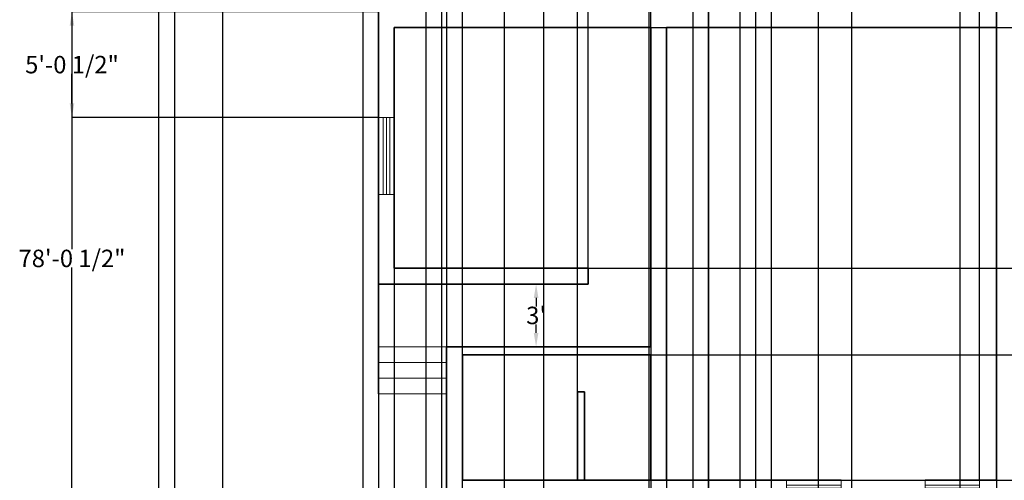
# Model space of a CAD drawing. Units: inches. Extents: x -63 to 800, y 3068 to 4133.
# Tile 2 of 5: x -63 to 501, y 3473 to 3737. Entities that reach past the tile are written whole.
import ezdxf

# ---------------------------------------------------------------- set-up
doc = ezdxf.new("R2010")
doc.units = ezdxf.units.IN
doc.header["$MEASUREMENT"] = 0
for name, color, linetype, lineweight in [('A-ANNO-DIMS', 2, 'Continuous', 13), ('A-FLOR-STRS', 3, 'Continuous', 18), ('A-GLAZ', 4, 'Continuous', 18), ('A-WALL', 7, 'Continuous', 35), ('A-WALL-SITE', 8, 'Continuous', 30)]:
    doc.layers.add(name, color=color, linetype=linetype, lineweight=lineweight)
doc.styles.get("Standard").update_dxf_attribs({"font": 'arial.ttf'})
doc.dimstyles.get("Standard").update_dxf_attribs({"dimtxt": 10, "dimasz": 8, "dimexe": 0.18, "dimexo": 0.0625, "dimgap": 0.09, "dimtad": 0, "dimtih": 1, "dimtoh": 1, "dimdec": 0, "dimzin": 0, "dimdsep": 46, "dimlunit": 3, "dimtxsty": 'Standard', "dimcen": 0.09, "dimadec": 0, "dimazin": 0, "dimtfac": 1, "dimtdec": 0, "dimtofl": 0, "dimtmove": 0, "dimatfit": 3, "dimfxl": 1, "dimtolj": 1, "dimtzin": 0, "dimarcsym": 0})

# ---------------------------------------------------------------- blocks, each defined once
blk = doc.blocks.new('*D6')
at = {"layer": 'A-ANNO-DIMS', "color": 0, "lineweight": -2, "transparency": 16777216}
for p, q in [((224.87, 3585.81), (232.74, 3585.81)), ((232.56, 3577.81), (232.56, 3573.01)), ((232.56, 3557.81), (232.56, 3562.61)), ((224.87, 3549.81), (232.74, 3549.81))]:
    blk.add_line(p, q, dxfattribs=at)
at = {"layer": 'A-ANNO-DIMS', "color": 0, "transparency": 16777216}
for points in [[(231.22, 3577.81), (233.89, 3577.81), (232.56, 3585.81)], [(231.22, 3557.81), (233.89, 3557.81), (232.56, 3549.81)]]:
    blk.add_solid(points, dxfattribs=at)
at = {"layer": 'Defpoints', "color": 0, "transparency": 16777216}
for p in [(224.81, 3585.81), (224.81, 3549.81), (232.56, 3549.81)]:
    blk.add_point(p, dxfattribs=at)
at = {"layer": 'A-ANNO-DIMS', "color": 0, "transparency": 16777216, "insert": (232.56, 3567.81), "char_height": 10, "attachment_point": 5}
blk.add_mtext("\\A1;3'", dxfattribs=at)
blk = doc.blocks.new('WIN-31')
blk.add_lwpolyline([(0, 9), (31.17, 9), (31.17, 0), (0, 0)], close=True)
blk.add_lwpolyline([(0, 4.5), (31.17, 4.5), (31.17, 6.29), (0, 6.29), (0, 2.51), (31.17, 2.51)])
blk = doc.blocks.new('WIN-44')
blk.add_lwpolyline([(0, 0), (0, 44.17), (9, 44.17), (9, 0)], close=True)
for points in [[(2.71, 44.17), (2.71, 0), (6.5, 0), (6.5, 44.17)], [(4.5, 0), (4.5, 44.17)]]:
    blk.add_lwpolyline(points)
blk = doc.blocks.new('*D20')
at = {"layer": 'A-ANNO-DIMS', "color": 0, "lineweight": -2, "transparency": 16777216}
for p, q in [((16.25, 4068.66), (-33.52, 4068.66)), ((-33.34, 4060.66), (-33.34, 3605.75)), ((-33.34, 3140.31), (-33.34, 3595.23)), ((16.25, 3132.31), (-33.52, 3132.31))]:
    blk.add_line(p, q, dxfattribs=at)
at = {"layer": 'A-ANNO-DIMS', "color": 0, "transparency": 16777216}
for points in [[(-34.67, 4060.66), (-32.01, 4060.66), (-33.34, 4068.66)], [(-34.67, 3140.31), (-32.01, 3140.31), (-33.34, 3132.31)]]:
    blk.add_solid(points, dxfattribs=at)
at = {"layer": 'Defpoints', "color": 0, "transparency": 16777216}
for p in [(-33.34, 4068.66), (16.31, 4068.66), (16.31, 3132.31)]:
    blk.add_point(p, dxfattribs=at)
at = {"layer": 'A-ANNO-DIMS', "color": 0, "transparency": 16777216, "insert": (-33.34, 3600.49), "char_height": 10, "attachment_point": 5}
blk.add_mtext('\\A1;78\'-0 1/2"', dxfattribs=at)
blk = doc.blocks.new('*D23')
at = {"layer": 'A-ANNO-DIMS', "color": 0, "lineweight": -2, "transparency": 16777216}
for p, q in [((25.31, 4059.6), (25.31, 3082.48)), ((169.31, 4059.6), (169.31, 3082.48)), ((33.31, 3082.66), (80.51, 3082.66)), ((161.31, 3082.66), (114.1, 3082.66))]:
    blk.add_line(p, q, dxfattribs=at)
at = {"layer": 'A-ANNO-DIMS', "color": 0, "transparency": 16777216}
for points in [[(33.31, 3083.99), (33.31, 3081.33), (25.31, 3082.66)], [(161.31, 3083.99), (161.31, 3081.33), (169.31, 3082.66)]]:
    blk.add_solid(points, dxfattribs=at)
at = {"layer": 'Defpoints', "color": 0, "transparency": 16777216}
for p in [(25.31, 4059.66), (169.31, 4059.66), (169.31, 3082.66)]:
    blk.add_point(p, dxfattribs=at)
at = {"layer": 'A-ANNO-DIMS', "color": 0, "transparency": 16777216, "insert": (97.31, 3082.66), "char_height": 10, "attachment_point": 5}
blk.add_mtext('\\A1;12\'-0"', dxfattribs=at)
blk = doc.blocks.new('*D24')
at = {"layer": 'A-ANNO-DIMS', "color": 0, "lineweight": -2, "transparency": 16777216}
for p, q in [((178.31, 4059.6), (178.31, 3082.48)), ((322.31, 4059.6), (322.31, 3082.48)), ((186.31, 3082.66), (233.51, 3082.66)), ((314.31, 3082.66), (267.1, 3082.66))]:
    blk.add_line(p, q, dxfattribs=at)
at = {"layer": 'A-ANNO-DIMS', "color": 0, "transparency": 16777216}
for points in [[(186.31, 3083.99), (186.31, 3081.33), (178.31, 3082.66)], [(314.31, 3083.99), (314.31, 3081.33), (322.31, 3082.66)]]:
    blk.add_solid(points, dxfattribs=at)
at = {"layer": 'Defpoints', "color": 0, "transparency": 16777216}
for p in [(178.31, 4059.66), (322.31, 4059.66), (322.31, 3082.66)]:
    blk.add_point(p, dxfattribs=at)
at = {"layer": 'A-ANNO-DIMS', "color": 0, "transparency": 16777216, "insert": (250.31, 3082.66), "char_height": 10, "attachment_point": 5}
blk.add_mtext('\\A1;12\'-0"', dxfattribs=at)
blk = doc.blocks.new('*D25')
at = {"layer": 'A-ANNO-DIMS', "color": 0, "lineweight": -2, "transparency": 16777216}
for p, q in [((331.31, 4059.6), (331.31, 3082.48)), ((475.31, 4059.6), (475.31, 3082.48)), ((339.31, 3082.66), (386.51, 3082.66)), ((467.31, 3082.66), (420.1, 3082.66))]:
    blk.add_line(p, q, dxfattribs=at)
at = {"layer": 'A-ANNO-DIMS', "color": 0, "transparency": 16777216}
for points in [[(339.31, 3083.99), (339.31, 3081.33), (331.31, 3082.66)], [(467.31, 3083.99), (467.31, 3081.33), (475.31, 3082.66)]]:
    blk.add_solid(points, dxfattribs=at)
at = {"layer": 'Defpoints', "color": 0, "transparency": 16777216}
for p in [(331.31, 4059.66), (475.31, 4059.66), (475.31, 3082.66)]:
    blk.add_point(p, dxfattribs=at)
at = {"layer": 'A-ANNO-DIMS', "color": 0, "transparency": 16777216, "insert": (403.31, 3082.66), "char_height": 10, "attachment_point": 5}
blk.add_mtext('\\A1;12\'-0"', dxfattribs=at)
blk = doc.blocks.new('*D27')
at = {"layer": 'A-ANNO-DIMS', "color": 0, "lineweight": -2, "transparency": 16777216}
for p, q in [((25.31, 3951.6), (25.31, 3082.48)), ((52.97, 3951.6), (52.97, 3082.48)), ((33.31, 3082.66), (44.97, 3082.66)), ((52.97, 3082.66), (60.97, 3082.66))]:
    blk.add_line(p, q, dxfattribs=at)
at = {"layer": 'A-ANNO-DIMS', "color": 0, "transparency": 16777216}
for points in [[(33.31, 3083.99), (33.31, 3081.33), (25.31, 3082.66)], [(44.97, 3083.99), (44.97, 3081.33), (52.97, 3082.66)]]:
    blk.add_solid(points, dxfattribs=at)
at = {"layer": 'Defpoints', "color": 0, "transparency": 16777216}
for p in [(25.31, 3951.66), (52.97, 3951.66), (52.97, 3082.66)]:
    blk.add_point(p, dxfattribs=at)
at = {"layer": 'A-ANNO-DIMS', "color": 0, "transparency": 16777216, "insert": (86.08, 3082.66), "char_height": 10, "attachment_point": 5}
blk.add_mtext('\\A1;2\'-3 1/2"', dxfattribs=at)
blk = doc.blocks.new('*D28')
at = {"layer": 'A-ANNO-DIMS', "color": 0, "lineweight": -2, "transparency": 16777216}
for p, q in [((297.16, 3951.55), (297.16, 3082.48)), ((331.31, 3951.6), (331.31, 3082.48)), ((305.16, 3082.66), (323.31, 3082.66)), ((331.31, 3082.66), (339.31, 3082.66))]:
    blk.add_line(p, q, dxfattribs=at)
at = {"layer": 'A-ANNO-DIMS', "color": 0, "transparency": 16777216}
for points in [[(305.16, 3083.99), (305.16, 3081.33), (297.16, 3082.66)], [(323.31, 3083.99), (323.31, 3081.33), (331.31, 3082.66)]]:
    blk.add_solid(points, dxfattribs=at)
at = {"layer": 'Defpoints', "color": 0, "transparency": 16777216}
for p in [(297.16, 3951.61), (331.31, 3951.66), (331.31, 3082.66)]:
    blk.add_point(p, dxfattribs=at)
at = {"layer": 'A-ANNO-DIMS', "color": 0, "transparency": 16777216, "insert": (356.66, 3082.66), "char_height": 10, "attachment_point": 5}
blk.add_mtext('\\A1;2\'-10"', dxfattribs=at)
blk = doc.blocks.new('*D29')
at = {"layer": 'A-ANNO-DIMS', "color": 0, "lineweight": -2, "transparency": 16777216}
for p, q in [((367.31, 3951.6), (367.31, 3082.48)), ((413.21, 3951.6), (413.21, 3082.48)), ((359.31, 3082.66), (351.31, 3082.66)), ((421.21, 3082.66), (429.21, 3082.66))]:
    blk.add_line(p, q, dxfattribs=at)
at = {"layer": 'A-ANNO-DIMS', "color": 0, "transparency": 16777216}
for points in [[(359.31, 3083.99), (359.31, 3081.33), (367.31, 3082.66)], [(421.21, 3083.99), (421.21, 3081.33), (413.21, 3082.66)]]:
    blk.add_solid(points, dxfattribs=at)
at = {"layer": 'Defpoints', "color": 0, "transparency": 16777216}
for p in [(367.31, 3951.66), (413.21, 3951.66), (413.21, 3082.66)]:
    blk.add_point(p, dxfattribs=at)
at = {"layer": 'A-ANNO-DIMS', "color": 0, "transparency": 16777216, "insert": (390.26, 3082.66), "char_height": 10, "attachment_point": 5}
blk.add_mtext('\\A1;3\'-10"', dxfattribs=at)
blk = doc.blocks.new('*D30')
at = {"layer": 'A-ANNO-DIMS', "color": 0, "lineweight": -2, "transparency": 16777216}
for p, q in [((133.31, 3951.6), (133.31, 3082.48)), ((169.31, 3951.6), (169.31, 3082.48)), ((125.31, 3082.66), (117.31, 3082.66)), ((177.31, 3082.66), (185.31, 3082.66))]:
    blk.add_line(p, q, dxfattribs=at)
at = {"layer": 'A-ANNO-DIMS', "color": 0, "transparency": 16777216}
for points in [[(125.31, 3083.99), (125.31, 3081.33), (133.31, 3082.66)], [(177.31, 3083.99), (177.31, 3081.33), (169.31, 3082.66)]]:
    blk.add_solid(points, dxfattribs=at)
at = {"layer": 'Defpoints', "color": 0, "transparency": 16777216}
for p in [(133.31, 3951.66), (169.31, 3951.66), (169.31, 3082.66)]:
    blk.add_point(p, dxfattribs=at)
at = {"layer": 'A-ANNO-DIMS', "color": 0, "transparency": 16777216, "insert": (151.31, 3082.66), "char_height": 10, "attachment_point": 5}
blk.add_mtext('\\A1;3\'-0"', dxfattribs=at)
blk = doc.blocks.new('*D31')
at = {"layer": 'A-ANNO-DIMS', "color": 0, "lineweight": -2, "transparency": 16777216}
for p, q in [((178.31, 3951.6), (178.31, 3082.48)), ((214.31, 3951.6), (214.31, 3082.48)), ((170.31, 3082.66), (162.31, 3082.66)), ((222.31, 3082.66), (230.31, 3082.66))]:
    blk.add_line(p, q, dxfattribs=at)
at = {"layer": 'A-ANNO-DIMS', "color": 0, "transparency": 16777216}
for points in [[(170.31, 3083.99), (170.31, 3081.33), (178.31, 3082.66)], [(222.31, 3083.99), (222.31, 3081.33), (214.31, 3082.66)]]:
    blk.add_solid(points, dxfattribs=at)
at = {"layer": 'Defpoints', "color": 0, "transparency": 16777216}
for p in [(178.31, 3951.66), (214.31, 3951.66), (214.31, 3082.66)]:
    blk.add_point(p, dxfattribs=at)
at = {"layer": 'A-ANNO-DIMS', "color": 0, "transparency": 16777216, "insert": (196.31, 3082.66), "char_height": 10, "attachment_point": 5}
blk.add_mtext('\\A1;3\'-0"', dxfattribs=at)
blk = doc.blocks.new('*D32')
at = {"layer": 'A-ANNO-DIMS', "color": 0, "lineweight": -2, "transparency": 16777216}
for p, q in [((331.31, 3951.6), (331.31, 3082.48)), ((367.31, 3951.6), (367.31, 3082.48)), ((323.31, 3082.66), (315.31, 3082.66)), ((375.31, 3082.66), (383.31, 3082.66))]:
    blk.add_line(p, q, dxfattribs=at)
at = {"layer": 'A-ANNO-DIMS', "color": 0, "transparency": 16777216}
for points in [[(323.31, 3083.99), (323.31, 3081.33), (331.31, 3082.66)], [(375.31, 3083.99), (375.31, 3081.33), (367.31, 3082.66)]]:
    blk.add_solid(points, dxfattribs=at)
at = {"layer": 'Defpoints', "color": 0, "transparency": 16777216}
for p in [(331.31, 3951.66), (367.31, 3951.66), (367.31, 3082.66)]:
    blk.add_point(p, dxfattribs=at)
at = {"layer": 'A-ANNO-DIMS', "color": 0, "transparency": 16777216, "insert": (349.31, 3082.66), "char_height": 10, "attachment_point": 5}
blk.add_mtext('\\A1;3\'-0"', dxfattribs=at)
blk = doc.blocks.new('*D34')
at = {"layer": 'A-ANNO-DIMS', "color": 0, "lineweight": -2, "transparency": 16777216}
for p, q in [((142.31, 3522.75), (142.31, 3082.48)), ((670.31, 3263.25), (670.31, 3082.48)), ((150.31, 3082.66), (388.84, 3082.66)), ((662.31, 3082.66), (423.78, 3082.66))]:
    blk.add_line(p, q, dxfattribs=at)
at = {"layer": 'A-ANNO-DIMS', "color": 0, "transparency": 16777216}
for points in [[(150.31, 3083.99), (150.31, 3081.33), (142.31, 3082.66)], [(662.31, 3083.99), (662.31, 3081.33), (670.31, 3082.66)]]:
    blk.add_solid(points, dxfattribs=at)
at = {"layer": 'Defpoints', "color": 0, "transparency": 16777216}
for p in [(142.31, 3522.81), (670.31, 3263.31), (670.31, 3082.66)]:
    blk.add_point(p, dxfattribs=at)
at = {"layer": 'A-ANNO-DIMS', "color": 0, "transparency": 16777216, "insert": (406.31, 3082.66), "char_height": 10, "attachment_point": 5}
blk.add_mtext('\\A1;44\'-0"', dxfattribs=at)
blk = doc.blocks.new('*D37')
at = {"layer": 'A-ANNO-DIMS', "color": 0, "lineweight": -2, "transparency": 16777216}
for p, q in [((181.31, 3885.75), (181.31, 3082.48)), ((349.31, 3885.75), (349.31, 3082.48)), ((189.31, 3082.66), (248.51, 3082.66)), ((341.31, 3082.66), (282.1, 3082.66))]:
    blk.add_line(p, q, dxfattribs=at)
at = {"layer": 'A-ANNO-DIMS', "color": 0, "transparency": 16777216}
for points in [[(189.31, 3083.99), (189.31, 3081.33), (181.31, 3082.66)], [(341.31, 3083.99), (341.31, 3081.33), (349.31, 3082.66)]]:
    blk.add_solid(points, dxfattribs=at)
at = {"layer": 'Defpoints', "color": 0, "transparency": 16777216}
for p in [(181.31, 3885.81), (349.31, 3885.81), (349.31, 3082.66)]:
    blk.add_point(p, dxfattribs=at)
at = {"layer": 'A-ANNO-DIMS', "color": 0, "transparency": 16777216, "insert": (265.31, 3082.66), "char_height": 10, "attachment_point": 5}
blk.add_mtext('\\A1;14\'-0"', dxfattribs=at)
blk = doc.blocks.new('*D38')
at = {"layer": 'A-ANNO-DIMS', "color": 0, "lineweight": -2, "transparency": 16777216}
for p, q in [((358.31, 3885.75), (358.31, 3082.48)), ((496.31, 3885.75), (496.31, 3082.48)), ((366.31, 3082.66), (410.51, 3082.66)), ((488.31, 3082.66), (444.1, 3082.66))]:
    blk.add_line(p, q, dxfattribs=at)
at = {"layer": 'A-ANNO-DIMS', "color": 0, "transparency": 16777216}
for points in [[(366.31, 3083.99), (366.31, 3081.33), (358.31, 3082.66)], [(488.31, 3083.99), (488.31, 3081.33), (496.31, 3082.66)]]:
    blk.add_solid(points, dxfattribs=at)
at = {"layer": 'Defpoints', "color": 0, "transparency": 16777216}
for p in [(358.31, 3885.81), (496.31, 3885.81), (496.31, 3082.66)]:
    blk.add_point(p, dxfattribs=at)
at = {"layer": 'A-ANNO-DIMS', "color": 0, "transparency": 16777216, "insert": (427.31, 3082.66), "char_height": 10, "attachment_point": 5}
blk.add_mtext('\\A1;11\'-6"', dxfattribs=at)
blk = doc.blocks.new('*D44')
at = {"layer": 'A-ANNO-DIMS', "color": 0, "lineweight": -2, "transparency": 16777216}
for p, q in [((151.31, 3732.75), (151.31, 3082.48)), ((298.31, 3732.75), (298.31, 3082.48)), ((159.31, 3082.66), (208.01, 3082.66)), ((290.31, 3082.66), (241.6, 3082.66))]:
    blk.add_line(p, q, dxfattribs=at)
at = {"layer": 'A-ANNO-DIMS', "color": 0, "transparency": 16777216}
for points in [[(159.31, 3083.99), (159.31, 3081.33), (151.31, 3082.66)], [(290.31, 3083.99), (290.31, 3081.33), (298.31, 3082.66)]]:
    blk.add_solid(points, dxfattribs=at)
at = {"layer": 'Defpoints', "color": 0, "transparency": 16777216}
for p in [(151.31, 3732.81), (298.31, 3732.81), (298.31, 3082.66)]:
    blk.add_point(p, dxfattribs=at)
at = {"layer": 'A-ANNO-DIMS', "color": 0, "transparency": 16777216, "insert": (224.81, 3082.66), "char_height": 10, "attachment_point": 5}
blk.add_mtext('\\A1;12\'-3"', dxfattribs=at)
blk = doc.blocks.new('*D45')
at = {"layer": 'A-ANNO-DIMS', "color": 0, "lineweight": -2, "transparency": 16777216}
for p, q in [((307.31, 3732.75), (307.31, 3082.48)), ((496.31, 3732.75), (496.31, 3082.48)), ((315.31, 3082.66), (385.01, 3082.66)), ((488.31, 3082.66), (418.6, 3082.66))]:
    blk.add_line(p, q, dxfattribs=at)
at = {"layer": 'A-ANNO-DIMS', "color": 0, "transparency": 16777216}
for points in [[(315.31, 3083.99), (315.31, 3081.33), (307.31, 3082.66)], [(488.31, 3083.99), (488.31, 3081.33), (496.31, 3082.66)]]:
    blk.add_solid(points, dxfattribs=at)
at = {"layer": 'Defpoints', "color": 0, "transparency": 16777216}
for p in [(307.31, 3732.81), (496.31, 3732.81), (496.31, 3082.66)]:
    blk.add_point(p, dxfattribs=at)
at = {"layer": 'A-ANNO-DIMS', "color": 0, "transparency": 16777216, "insert": (401.81, 3082.66), "char_height": 10, "attachment_point": 5}
blk.add_mtext('\\A1;15\'-9"', dxfattribs=at)
blk = doc.blocks.new('*D47')
at = {"layer": 'A-ANNO-DIMS', "color": 0, "lineweight": -2, "transparency": 16777216}
for p, q in [((151.37, 3732.81), (771.14, 3732.81)), ((770.96, 3724.81), (770.96, 3669.01)), ((770.96, 3602.81), (770.96, 3658.61)), ((151.37, 3594.81), (771.14, 3594.81))]:
    blk.add_line(p, q, dxfattribs=at)
at = {"layer": 'A-ANNO-DIMS', "color": 0, "transparency": 16777216}
for points in [[(769.63, 3724.81), (772.29, 3724.81), (770.96, 3732.81)], [(769.63, 3602.81), (772.29, 3602.81), (770.96, 3594.81)]]:
    blk.add_solid(points, dxfattribs=at)
at = {"layer": 'Defpoints', "color": 0, "transparency": 16777216}
for p in [(151.31, 3732.81), (770.96, 3732.81), (151.31, 3594.81)]:
    blk.add_point(p, dxfattribs=at)
at = {"layer": 'A-ANNO-DIMS', "color": 0, "transparency": 16777216, "insert": (770.96, 3663.81), "char_height": 10, "attachment_point": 5}
blk.add_mtext('\\A1;11\'-6"', dxfattribs=at)
blk = doc.blocks.new('*D48')
at = {"layer": 'A-ANNO-DIMS', "color": 0, "lineweight": -2, "transparency": 16777216}
for p, q in [((307.37, 3732.81), (771.14, 3732.81)), ((770.96, 3724.81), (770.96, 3608.32)), ((770.96, 3481.31), (770.96, 3597.8)), ((307.37, 3473.31), (771.14, 3473.31))]:
    blk.add_line(p, q, dxfattribs=at)
at = {"layer": 'A-ANNO-DIMS', "color": 0, "transparency": 16777216}
for points in [[(769.63, 3724.81), (772.29, 3724.81), (770.96, 3732.81)], [(769.63, 3481.31), (772.29, 3481.31), (770.96, 3473.31)]]:
    blk.add_solid(points, dxfattribs=at)
at = {"layer": 'Defpoints', "color": 0, "transparency": 16777216}
for p in [(307.31, 3732.81), (770.96, 3732.81), (307.31, 3473.31)]:
    blk.add_point(p, dxfattribs=at)
at = {"layer": 'A-ANNO-DIMS', "color": 0, "transparency": 16777216, "insert": (770.96, 3603.06), "char_height": 10, "attachment_point": 5}
blk.add_mtext('\\A1;21\'-7 1/2"', dxfattribs=at)
blk = doc.blocks.new('*D49')
at = {"layer": 'A-ANNO-DIMS', "color": 0, "lineweight": -2, "transparency": 16777216}
for p, q in [((142.25, 3741.81), (-33.52, 3741.81)), ((-33.34, 3733.81), (-33.34, 3716.81)), ((-33.34, 3689.29), (-33.34, 3706.29)), ((142.25, 3681.29), (-33.52, 3681.29))]:
    blk.add_line(p, q, dxfattribs=at)
at = {"layer": 'A-ANNO-DIMS', "color": 0, "transparency": 16777216}
for points in [[(-34.67, 3733.81), (-32.01, 3733.81), (-33.34, 3741.81)], [(-34.67, 3689.29), (-32.01, 3689.29), (-33.34, 3681.29)]]:
    blk.add_solid(points, dxfattribs=at)
at = {"layer": 'Defpoints', "color": 0, "transparency": 16777216}
for p in [(-33.34, 3741.81), (142.31, 3741.81), (142.31, 3681.29)]:
    blk.add_point(p, dxfattribs=at)
at = {"layer": 'A-ANNO-DIMS', "color": 0, "transparency": 16777216, "insert": (-33.34, 3711.55), "char_height": 10, "attachment_point": 5}
blk.add_mtext('\\A1;5\'-0 1/2"', dxfattribs=at)
blk = doc.blocks.new('*D57')
at = {"layer": 'A-ANNO-DIMS', "color": 0, "lineweight": -2, "transparency": 16777216}
for p, q in [((190.31, 3311.37), (190.31, 4118.49)), ((198.31, 4118.31), (228.97, 4118.31)), ((236.97, 3320.37), (236.97, 4118.49)), ((236.97, 4118.31), (244.97, 4118.31))]:
    blk.add_line(p, q, dxfattribs=at)
at = {"layer": 'A-ANNO-DIMS', "color": 0, "transparency": 16777216}
for points in [[(198.31, 4119.64), (198.31, 4116.98), (190.31, 4118.31)], [(228.97, 4119.64), (228.97, 4116.98), (236.97, 4118.31)]]:
    blk.add_solid(points, dxfattribs=at)
at = {"layer": 'Defpoints', "color": 0, "transparency": 16777216}
for p in [(236.97, 4118.31), (236.97, 3320.31), (190.31, 3311.31)]:
    blk.add_point(p, dxfattribs=at)
at = {"layer": 'A-ANNO-DIMS', "color": 0, "transparency": 16777216, "insert": (273.88, 4118.31), "char_height": 10, "attachment_point": 5}
blk.add_mtext('\\A1;3\'-10 1/2"', dxfattribs=at)
blk = doc.blocks.new('*D62')
at = {"layer": 'A-ANNO-DIMS', "color": 0, "lineweight": -2, "transparency": 16777216}
for p, q in [((478.66, 4118.31), (470.66, 4118.31)), ((486.66, 3473.37), (486.66, 4118.49)), ((496.31, 3473.37), (496.31, 4118.49)), ((504.31, 4118.31), (512.31, 4118.31))]:
    blk.add_line(p, q, dxfattribs=at)
at = {"layer": 'A-ANNO-DIMS', "color": 0, "transparency": 16777216}
for points in [[(478.66, 4119.64), (478.66, 4116.98), (486.66, 4118.31)], [(504.31, 4119.64), (504.31, 4116.98), (496.31, 4118.31)]]:
    blk.add_solid(points, dxfattribs=at)
at = {"layer": 'Defpoints', "color": 0, "transparency": 16777216}
for p in [(496.31, 4118.31), (486.66, 3473.31), (496.31, 3473.31)]:
    blk.add_point(p, dxfattribs=at)
at = {"layer": 'A-ANNO-DIMS', "color": 0, "transparency": 16777216, "insert": (537.34, 4118.31), "char_height": 10, "attachment_point": 5}
blk.add_mtext('\\A1;0\'-9 1/2"', dxfattribs=at)
blk = doc.blocks.new('*D63')
at = {"layer": 'A-ANNO-DIMS', "color": 0, "lineweight": -2, "transparency": 16777216}
for p, q in [((190.37, 3545.31), (771.14, 3545.31)), ((770.96, 3537.31), (770.96, 3514.51)), ((770.96, 3481.31), (770.96, 3504.11)), ((190.37, 3473.31), (771.14, 3473.31))]:
    blk.add_line(p, q, dxfattribs=at)
at = {"layer": 'A-ANNO-DIMS', "color": 0, "transparency": 16777216}
for points in [[(769.63, 3537.31), (772.29, 3537.31), (770.96, 3545.31)], [(769.63, 3481.31), (772.29, 3481.31), (770.96, 3473.31)]]:
    blk.add_solid(points, dxfattribs=at)
at = {"layer": 'Defpoints', "color": 0, "transparency": 16777216}
for p in [(190.31, 3545.31), (770.96, 3545.31), (190.31, 3473.31)]:
    blk.add_point(p, dxfattribs=at)
at = {"layer": 'A-ANNO-DIMS', "color": 0, "transparency": 16777216, "insert": (770.96, 3509.31), "char_height": 10, "attachment_point": 5}
blk.add_mtext('\\A1;6\'-0"', dxfattribs=at)
blk = doc.blocks.new('*D64')
at = {"layer": 'A-ANNO-DIMS', "color": 0, "lineweight": -2, "transparency": 16777216}
for p, q in [((190.31, 3473.37), (190.31, 4118.49)), ((198.31, 4118.31), (209.93, 4118.31)), ((248.31, 4118.31), (236.69, 4118.31)), ((256.31, 3473.37), (256.31, 4118.49))]:
    blk.add_line(p, q, dxfattribs=at)
at = {"layer": 'A-ANNO-DIMS', "color": 0, "transparency": 16777216}
for points in [[(198.31, 4119.64), (198.31, 4116.98), (190.31, 4118.31)], [(248.31, 4119.64), (248.31, 4116.98), (256.31, 4118.31)]]:
    blk.add_solid(points, dxfattribs=at)
at = {"layer": 'Defpoints', "color": 0, "transparency": 16777216}
for p in [(256.31, 4118.31), (190.31, 3473.31), (256.31, 3473.31)]:
    blk.add_point(p, dxfattribs=at)
at = {"layer": 'A-ANNO-DIMS', "color": 0, "transparency": 16777216, "insert": (223.31, 4118.31), "char_height": 10, "attachment_point": 5}
blk.add_mtext('\\A1;5\'-6"', dxfattribs=at)
blk = doc.blocks.new('*D68')
at = {"layer": 'A-ANNO-DIMS', "color": 0, "lineweight": -2, "transparency": 16777216}
for p, q in [((254.31, 4118.31), (246.31, 4118.31)), ((262.31, 3594.87), (262.31, 4118.49)), ((298.31, 3549.87), (298.31, 4118.49)), ((306.31, 4118.31), (314.31, 4118.31))]:
    blk.add_line(p, q, dxfattribs=at)
at = {"layer": 'A-ANNO-DIMS', "color": 0, "transparency": 16777216}
for points in [[(254.31, 4119.64), (254.31, 4116.98), (262.31, 4118.31)], [(306.31, 4119.64), (306.31, 4116.98), (298.31, 4118.31)]]:
    blk.add_solid(points, dxfattribs=at)
at = {"layer": 'Defpoints', "color": 0, "transparency": 16777216}
for p in [(298.31, 4118.31), (262.31, 3594.81), (298.31, 3549.81)]:
    blk.add_point(p, dxfattribs=at)
at = {"layer": 'A-ANNO-DIMS', "color": 0, "transparency": 16777216, "insert": (280.31, 4118.31), "char_height": 10, "attachment_point": 5}
blk.add_mtext('\\A1;3\'-0"', dxfattribs=at)
blk = doc.blocks.new('*D69')
at = {"layer": 'A-ANNO-DIMS', "color": 0, "lineweight": -2, "transparency": 16777216}
for p, q in [((142.31, 3522.75), (142.31, 3082.48)), ((181.31, 3522.75), (181.31, 3082.48)), ((134.31, 3082.66), (126.31, 3082.66)), ((189.31, 3082.66), (197.31, 3082.66))]:
    blk.add_line(p, q, dxfattribs=at)
at = {"layer": 'A-ANNO-DIMS', "color": 0, "transparency": 16777216}
for points in [[(134.31, 3083.99), (134.31, 3081.33), (142.31, 3082.66)], [(189.31, 3083.99), (189.31, 3081.33), (181.31, 3082.66)]]:
    blk.add_solid(points, dxfattribs=at)
at = {"layer": 'Defpoints', "color": 0, "transparency": 16777216}
for p in [(142.31, 3522.81), (181.31, 3522.81), (181.31, 3082.66)]:
    blk.add_point(p, dxfattribs=at)
at = {"layer": 'A-ANNO-DIMS', "color": 0, "transparency": 16777216, "insert": (161.81, 3082.66), "char_height": 10, "attachment_point": 5}
blk.add_mtext('\\A1;3\'-3"', dxfattribs=at)
blk = doc.blocks.new('*D70')
at = {"layer": 'A-ANNO-DIMS', "color": 0, "lineweight": -2, "transparency": 16777216}
for p, q in [((331.31, 3263.37), (331.31, 4118.49)), ((339.31, 4118.31), (349.43, 4118.31)), ((386.31, 4118.31), (376.19, 4118.31)), ((394.31, 3263.37), (394.31, 4118.49))]:
    blk.add_line(p, q, dxfattribs=at)
at = {"layer": 'A-ANNO-DIMS', "color": 0, "transparency": 16777216}
for points in [[(339.31, 4119.64), (339.31, 4116.98), (331.31, 4118.31)], [(386.31, 4119.64), (386.31, 4116.98), (394.31, 4118.31)]]:
    blk.add_solid(points, dxfattribs=at)
at = {"layer": 'Defpoints', "color": 0, "transparency": 16777216}
for p in [(394.31, 4118.31), (331.31, 3263.31), (394.31, 3263.31)]:
    blk.add_point(p, dxfattribs=at)
at = {"layer": 'A-ANNO-DIMS', "color": 0, "transparency": 16777216, "insert": (362.81, 4118.31), "char_height": 10, "attachment_point": 5}
blk.add_mtext('\\A1;5\'-3"', dxfattribs=at)

msp = doc.modelspace()

# ---------------------------------------------------------------- linework, layer by layer
at = {"layer": 'A-FLOR-STRS'}
for p, q in [((181.31, 3549.81), (142.31, 3549.81)), ((181.31, 3540.81), (142.31, 3540.81)), ((181.31, 3531.81), (142.31, 3531.81)), ((181.31, 3522.81), (142.31, 3522.81))]:
    msp.add_line(p, q, dxfattribs=at)
at = {"layer": 'A-WALL'}
for p, q in [((142.31, 3741.81), (142.31, 3522.81)), ((151.31, 3732.81), (298.31, 3732.81)), ((151.31, 3732.81), (151.31, 3594.81)), ((298.31, 3732.81), (298.31, 3594.81)), ((307.31, 3732.81), (307.31, 3473.31)), ((307.31, 3732.81), (496.31, 3732.81)), ((496.31, 3732.81), (496.31, 3473.31)), ((151.31, 3594.81), (262.31, 3594.81)), ((142.31, 3585.81), (262.31, 3585.81)), ((298.31, 3585.81), (298.31, 3549.81)), ((181.31, 3549.81), (298.31, 3549.81)), ((181.31, 3549.81), (181.31, 3311.31)), ((190.31, 3545.31), (256.31, 3545.31)), ((190.31, 3545.31), (190.31, 3473.31)), ((260.31, 3545.31), (298.31, 3545.31)), ((298.31, 3545.31), (298.31, 3473.31)), ((256.31, 3523.99), (256.31, 3473.31)), ((260.31, 3523.99), (260.31, 3473.31)), ((190.31, 3473.31), (407.28, 3473.31)), ((455.48, 3473.31), (496.31, 3473.31))]:
    msp.add_line(p, q, dxfattribs=at)
for points in [[(262.31, 3585.81), (262.31, 3594.81)], [(298.31, 3596.81), (298.31, 3596.81), (298.31, 3585.81)], [(249.31, 3545.31), (260.31, 3545.31)], [(260.31, 3523.99), (256.31, 3523.99)]]:
    msp.add_lwpolyline(points, dxfattribs=at)
at = {"layer": 'A-WALL-SITE'}
for p, q in [((16.31, 4068.66), (16.31, 3132.31)), ((25.31, 3951.66), (25.31, 3132.31))]:
    msp.add_line(p, q, dxfattribs=at)

# ---------------------------------------------------------------- block references
at = {"layer": 'A-GLAZ'}
for name, p in [('WIN-44', (142.31, 3637.11)), ('WIN-31', (376.11, 3464.31)), ('WIN-31', (455.48, 3464.31))]:
    msp.add_blockref(name, p, dxfattribs=at)

# ---------------------------------------------------------------- dimensions: what is measured, and where the dimension line sits
at = {"layer": 'A-ANNO-DIMS'}
for base, p1, p2, picture, middle in [((236.97, 4118.31), (190.31, 3311.31), (236.97, 3320.31), '*D57', (273.88, 4118.31)), ((496.3095, 4118.3113), (486.6577, 3473.3102), (496.3095, 3473.3102), '*D62', (537.3415, 4118.3113)), ((256.31, 4118.31), (190.31, 3473.31), (256.31, 3473.31), '*D64', (223.31, 4118.31)), ((298.31, 4118.31), (262.31, 3594.81), (298.31, 3549.81), '*D68', (280.31, 4118.31)), ((394.31, 4118.31), (331.31, 3263.31), (394.31, 3263.31), '*D70', (362.81, 4118.31)), ((169.31, 3082.66), (25.31, 4059.66), (169.31, 4059.66), '*D23', (97.31, 3082.66)), ((322.31, 3082.66), (178.31, 4059.66), (322.31, 4059.66), '*D24', (250.31, 3082.66)), ((475.31, 3082.66), (331.31, 4059.66), (475.31, 4059.66), '*D25', (403.31, 3082.66)), ((52.97, 3082.66), (25.31, 3951.66), (52.97, 3951.66), '*D27', (86.08, 3082.66)), ((169.31, 3082.66), (133.31, 3951.66), (169.31, 3951.66), '*D30', (151.31, 3082.66)), ((214.31, 3082.66), (178.31, 3951.66), (214.31, 3951.66), '*D31', (196.31, 3082.66)), ((331.3095, 3082.6602), (297.1617, 3951.6131), (331.3095, 3951.6613), '*D28', (356.6607, 3082.6602)), ((367.31, 3082.66), (331.31, 3951.66), (367.31, 3951.66), '*D32', (349.31, 3082.66)), ((413.21, 3082.66), (367.31, 3951.66), (413.21, 3951.66), '*D29', (390.26, 3082.66)), ((349.31, 3082.66), (181.31, 3885.81), (349.31, 3885.81), '*D37', (265.31, 3082.66)), ((496.31, 3082.66), (358.31, 3885.81), (496.31, 3885.81), '*D38', (427.31, 3082.66)), ((298.31, 3082.66), (151.31, 3732.81), (298.31, 3732.81), '*D44', (224.81, 3082.66)), ((496.31, 3082.66), (307.31, 3732.81), (496.31, 3732.81), '*D45', (401.81, 3082.66)), ((181.31, 3082.66), (142.31, 3522.81), (181.31, 3522.81), '*D69', (161.81, 3082.66)), ((670.31, 3082.66), (142.31, 3522.81), (670.31, 3263.31), '*D34', (406.31, 3082.66))]:
    dim = msp.add_linear_dim(base=base, p1=p1, p2=p2, dimstyle='Standard', override={"dimdec": 1, "dimlfac": 1, "dimrnd": 0, "dimzin": 1, "dimdsep": 46, "dimlunit": 4, "dimfrac": 2}, dxfattribs=at)
    dim.commit()
    dim.dimension.update_dxf_attribs({"geometry": picture, "text_midpoint": middle})
for base, p1, p2, override, picture, middle in [((-33.3405, 4068.6613), (16.3095, 3132.3102), (16.3095, 4068.6613), {"dimdec": 1, "dimlfac": 1, "dimrnd": 0, "dimzin": 1, "dimdsep": 46, "dimlunit": 4, "dimfrac": 2}, '*D20', (-33.3405, 3600.4858)), ((-33.34, 3741.81), (142.31, 3681.29), (142.31, 3741.81), {"dimdec": 1, "dimlfac": 1, "dimrnd": 0, "dimzin": 1, "dimdsep": 46, "dimlunit": 4, "dimfrac": 2}, '*D49', (-33.34, 3711.55)), ((770.96, 3732.81), (151.31, 3594.81), (151.31, 3732.81), {"dimdec": 1, "dimlfac": 1, "dimrnd": 0, "dimzin": 1, "dimdsep": 46, "dimlunit": 4, "dimfrac": 2}, '*D47', (770.96, 3663.81)), ((770.96, 3732.81), (307.31, 3473.31), (307.31, 3732.81), {"dimdec": 1, "dimlfac": 1, "dimrnd": 0, "dimzin": 1, "dimdsep": 46, "dimlunit": 4, "dimfrac": 2}, '*D48', (770.96, 3603.06)), ((232.56, 3549.81), (224.81, 3585.81), (224.81, 3549.81), {"dimclrd": 0, "dimclre": 0, "dimclrt": 0}, '*D6', (232.56, 3567.81)), ((770.96, 3545.31), (190.31, 3473.31), (190.31, 3545.31), {"dimdec": 1, "dimlfac": 1, "dimrnd": 0, "dimzin": 1, "dimdsep": 46, "dimlunit": 4, "dimfrac": 2}, '*D63', (770.96, 3509.31))]:
    dim = msp.add_linear_dim(base=base, p1=p1, p2=p2, angle=90, dimstyle='Standard', override=override, dxfattribs=at)
    dim.commit()
    dim.dimension.update_dxf_attribs({"geometry": picture, "text_midpoint": middle})

doc.saveas('drawing.dxf')
